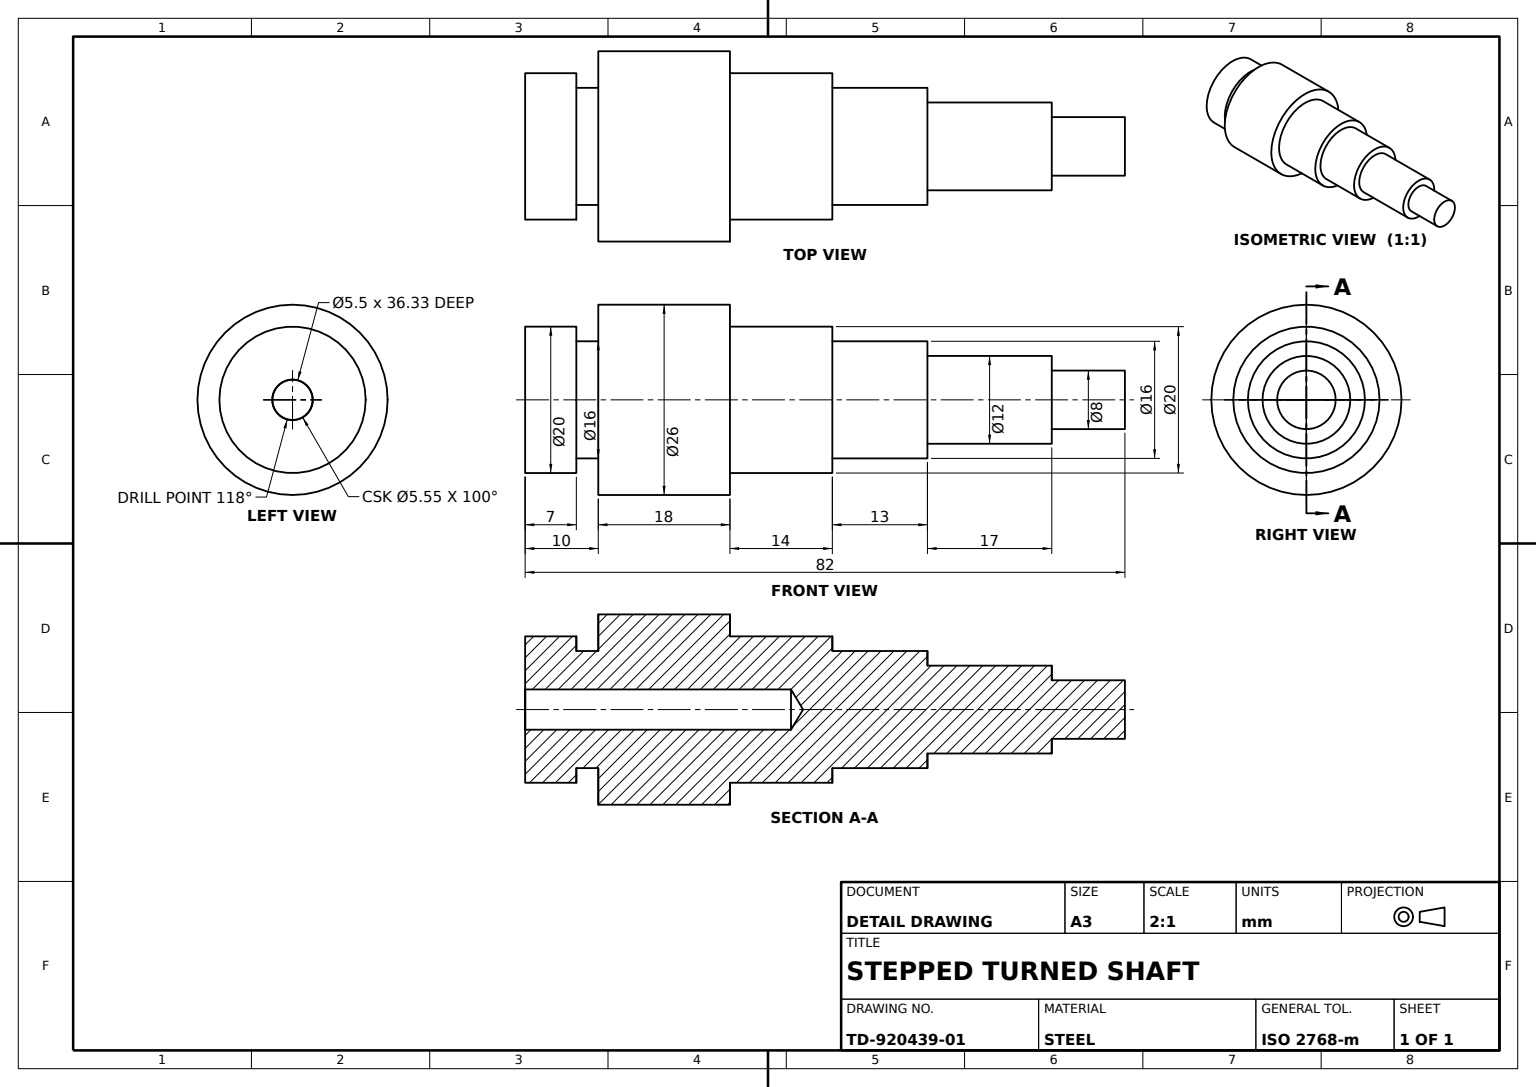
from build123d import *

# Parameters (mm, degrees)
AXIAL_HOLE_M5_CLEARANCE_D           = 5.5
AXIAL_HOLE_M5_CLEARANCE_DEPTH       = 36.347633298
AXIAL_HOLE_M5_CLEARANCE_CSINK_D     = 5.55
AXIAL_HOLE_M5_CLEARANCE_CSINK_ANGLE = 100
AXIAL_HOLE_M5_CLEARANCE_TIP         = 1.652366702


with BuildPart() as part:
    # Shaft Profile Sketch → Stepped Shaft Revolve (revolve)
    with BuildSketch(Plane.XY, mode=Mode.PRIVATE) as stepped_shaft_revolve_sk:
        Polygon((0, 0), (0, 10), (7, 10), (7, 8), (10, 8), (10, 13), (28, 13), (28, 10), (42, 10), (42, 8), (55, 8), (55, 6), (72, 6), (72, 4), (82, 4), (82, 0), align=None)
    revolve(stepped_shaft_revolve_sk.sketch.rotate(Axis((-602.792603174, 0, 0), (1, 0, 0)), 90), axis=Axis((-602.792603174, 0, 0), (1, 0, 0)))

    # Axial Hole M5 Clearance
    with Locations(Plane(origin=(0, 0, 0), x_dir=(0, 0, -1), z_dir=(-1, 0, 0))):
        with Locations((0, 0)):
            CounterSinkHole(AXIAL_HOLE_M5_CLEARANCE_D / 2, AXIAL_HOLE_M5_CLEARANCE_CSINK_D / 2, depth=AXIAL_HOLE_M5_CLEARANCE_DEPTH, counter_sink_angle=AXIAL_HOLE_M5_CLEARANCE_CSINK_ANGLE)
            with Locations((0, 0, -(AXIAL_HOLE_M5_CLEARANCE_DEPTH + AXIAL_HOLE_M5_CLEARANCE_TIP / 2))):  # 118° drill point
                Cone(0, AXIAL_HOLE_M5_CLEARANCE_D / 2, AXIAL_HOLE_M5_CLEARANCE_TIP, mode=Mode.SUBTRACT)


solid = part.part
